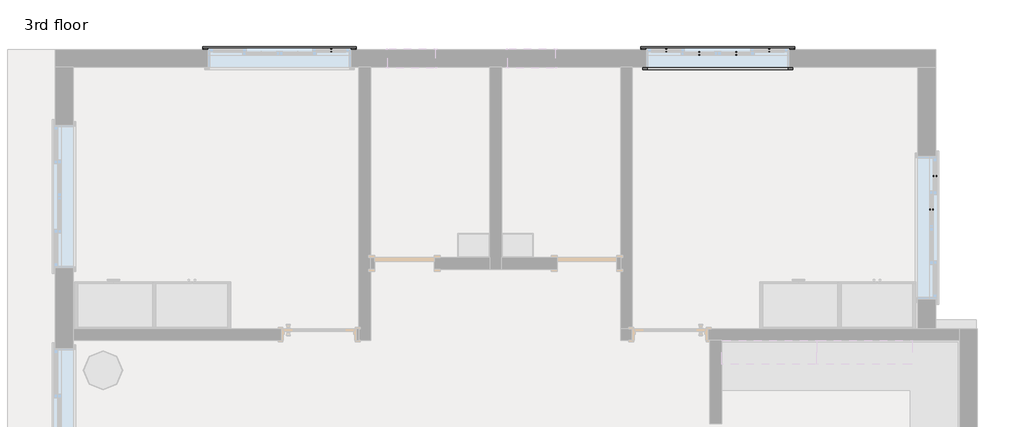
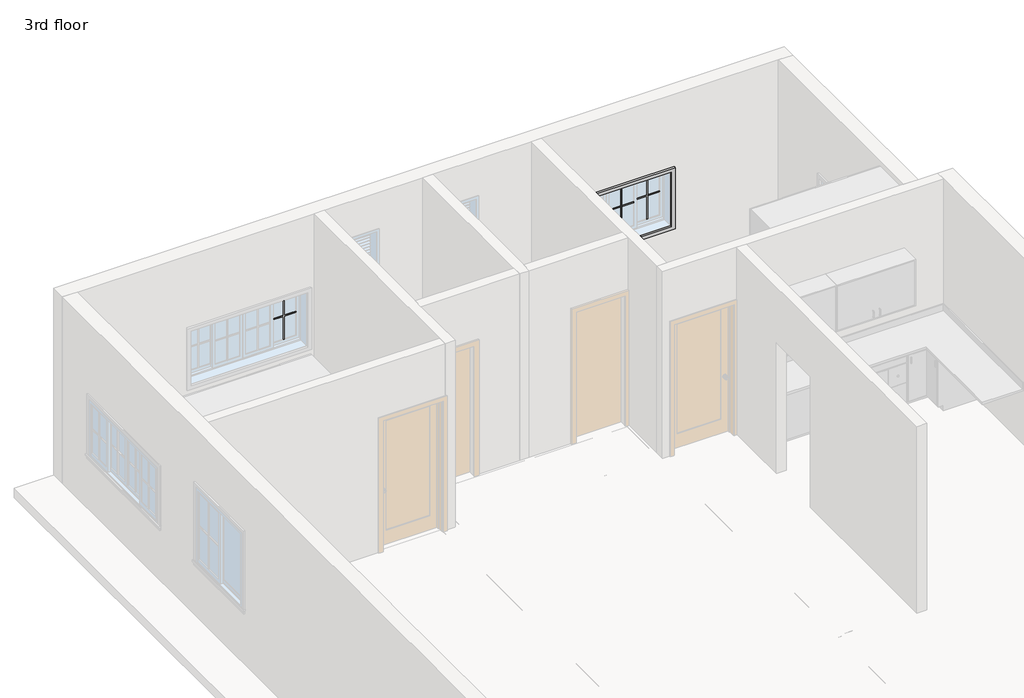
# One storey, part 4 of 4: 10 proxies.
"""IFC4 building model written with IfcOpenShell, lengths in millimetres."""

from ifc_helpers import new_model, si_unit, origin, place, context, project, spatial, transform, mapped, element, save
from components import muntin_pattern_2x2_muntin_pattern_2x2_31a16349, trim_window_exterior_flat_with_sill_3c945769, trim_window_interior_flat_picture_frame_0edfbaa2

model = new_model("IFC4")

# Units and contexts
model_context = context("Model", 3, world=origin())
ifc_project = project(units=[si_unit("LENGTHUNIT", "METRE", prefix="MILLI")], contexts=[model_context])

# Site, building, storey
site = spatial("IfcSite", under=ifc_project)
building = spatial("IfcBuilding", under=site)
storey = spatial("IfcBuildingStorey", under=building, Name="3rd floor", Elevation=10210.8)

# Proxies
placement = place(None, origin())
muntin_pattern_2x2_muntin_pattern_2x2_shape = muntin_pattern_2x2_muntin_pattern_2x2_31a16349(model_context)
element("IfcBuildingElementProxy", 1, Name="Muntin Pattern_2x2 : Muntin Pattern_2x2", ObjectType="Muntin Pattern_2x2 : Muntin Pattern_2x2", at=placement, inside=storey, context=model_context, shape_type="MappedRepresentation", body=[
    mapped(muntin_pattern_2x2_muntin_pattern_2x2_shape, transform((-9111.6124084, 10171.2711804, 11207.75), x_axis=(1.0, 0.0, 0.0), y_axis=(0.0, 1.0, 0.0), z_axis=(0.0, 0.0, 1.0))),
])
element("IfcBuildingElementProxy", 2, Name="Muntin Pattern_2x2 : Muntin Pattern_2x2", ObjectType="Muntin Pattern_2x2 : Muntin Pattern_2x2", at=placement, inside=storey, context=model_context, shape_type="MappedRepresentation", body=[
    mapped(muntin_pattern_2x2_muntin_pattern_2x2_shape, transform((-1374.1374084, 8555.1961804, 11207.75), x_axis=(0.0, -1.0, 0.0), y_axis=(1.0, 0.0, 0.0), z_axis=(0.0, 0.0, 1.0))),
])
element("IfcBuildingElementProxy", 3, Name="Muntin Pattern_2x2 : Muntin Pattern_2x2", ObjectType="Muntin Pattern_2x2 : Muntin Pattern_2x2", at=placement, inside=storey, context=model_context, shape_type="MappedRepresentation", body=[
    mapped(muntin_pattern_2x2_muntin_pattern_2x2_shape, transform((-1418.5874084, 8129.7461804, 11207.75), x_axis=(0.0, -1.0, 0.0), y_axis=(1.0, 0.0, 0.0), z_axis=(0.0, 0.0, 1.0))),
])
element("IfcBuildingElementProxy", 4, Name="Muntin Pattern_2x2 : Muntin Pattern_2x2", ObjectType="Muntin Pattern_2x2 : Muntin Pattern_2x2", at=placement, inside=storey, context=model_context, shape_type="MappedRepresentation", body=[
    mapped(muntin_pattern_2x2_muntin_pattern_2x2_shape, transform((-4819.0124084, 10171.2711804, 11207.75), x_axis=(1.0, 0.0, 0.0), y_axis=(0.0, 1.0, 0.0), z_axis=(0.0, 0.0, 1.0))),
])
element("IfcBuildingElementProxy", 5, Name="Muntin Pattern_2x2 : Muntin Pattern_2x2", ObjectType="Muntin Pattern_2x2 : Muntin Pattern_2x2", at=placement, inside=storey, context=model_context, shape_type="MappedRepresentation", body=[
    mapped(muntin_pattern_2x2_muntin_pattern_2x2_shape, transform((-4393.5624084, 10126.8211804, 11207.75), x_axis=(1.0, 0.0, 0.0), y_axis=(0.0, 1.0, 0.0), z_axis=(0.0, 0.0, 1.0))),
])
element("IfcBuildingElementProxy", 6, Name="Muntin Pattern_2x2 : Muntin Pattern_2x2", ObjectType="Muntin Pattern_2x2 : Muntin Pattern_2x2", at=placement, inside=storey, context=model_context, shape_type="MappedRepresentation", body=[
    mapped(muntin_pattern_2x2_muntin_pattern_2x2_shape, transform((-3923.6624084, 10126.8211804, 11207.75), x_axis=(1.0, 0.0, 0.0), y_axis=(0.0, 1.0, 0.0), z_axis=(0.0, 0.0, 1.0))),
])
element("IfcBuildingElementProxy", 7, Name="Muntin Pattern_2x2 : Muntin Pattern_2x2", ObjectType="Muntin Pattern_2x2 : Muntin Pattern_2x2", at=placement, inside=storey, context=model_context, shape_type="MappedRepresentation", body=[
    mapped(muntin_pattern_2x2_muntin_pattern_2x2_shape, transform((-3498.2124084, 10171.2711804, 11207.75), x_axis=(1.0, 0.0, 0.0), y_axis=(0.0, 1.0, 0.0), z_axis=(0.0, 0.0, 1.0))),
])
trim_window_exterior_flat_with_sill_shape = trim_window_exterior_flat_with_sill_3c945769(model_context)
element("IfcBuildingElementProxy", 8, Name="Trim-Window-Exterior-Flat : with Sill", ObjectType="Trim-Window-Exterior-Flat : with Sill", at=placement, inside=storey, context=model_context, shape_type="MappedRepresentation", body=[
    mapped(trim_window_exterior_flat_with_sill_shape, transform((-9772.0124084, 10180.7961804, 12039.6), x_axis=(-1.0, 0.0, 0.0), y_axis=(0.0, 0.0, 1.0), z_axis=(0.0, 1.0, 0.0))),
])
element("IfcBuildingElementProxy", 9, Name="Trim-Window-Exterior-Flat : with Sill", ObjectType="Trim-Window-Exterior-Flat : with Sill", at=placement, inside=storey, context=model_context, shape_type="MappedRepresentation", body=[
    mapped(trim_window_exterior_flat_with_sill_shape, transform((-4158.6124084, 10180.7961804, 12039.6), x_axis=(-1.0, 0.0, 0.0), y_axis=(0.0, 0.0, 1.0), z_axis=(0.0, 1.0, 0.0))),
])
trim_window_interior_flat_picture_frame_shape = trim_window_interior_flat_picture_frame_0edfbaa2(model_context)
element("IfcBuildingElementProxy", 10, Name="Trim-Window-Interior-Flat : Picture Frame", ObjectType="Trim-Window-Interior-Flat : Picture Frame", at=placement, inside=storey, context=model_context, shape_type="MappedRepresentation", body=[
    mapped(trim_window_interior_flat_picture_frame_shape, transform((-4158.6124084, 9952.1961804, 12039.6), x_axis=(1.0, 0.0, 0.0), y_axis=(0.0, 0.0, 1.0), z_axis=(0.0, -1.0, 0.0))),
])

save(model, "model.ifc")

# Revit data of these elements
# Type "Muntin Pattern_2x2 : Muntin Pattern_2x2"
#   Width [instance default] = 4' - 0"
#   Thickness = 0' - 0 1/2"
#   Height [instance default] = 4' - 0"
#   Distance = 0' - 0 3/4"
#   Interior Material [instance default] = none
#   Exterior Material [instance default] = none
#   Default Elevation = 0
# Type "Trim-Window-Exterior-Flat : with Sill"
#   Trim Width = 0' - 2 1/4"
#   Trim Thickness_Picture Frame = 0' - 1 1/4"
#   Trim Thickness_with Sill = 0' - 0 3/4"
#   Sill Thickness = 0' - 1 1/4"
#   Opening Width [instance default] = 2' - 0"
#   Opening Height [instance default] = 3' - 0"
#   Default Elevation = 4' - 0"
#   Sill = yes
#   Picture Frame = no
#   Trim Material [instance default] = none
# Type "Trim-Window-Interior-Flat : Picture Frame"
#   Trim Thickness_Picture Frame = 0' - 1 1/4"
#   Trim Width = 0' - 2 1/4"
#   Trim Thickness_with Sill = 0' - 0 3/4"
#   Sill Thickness = 0' - 1 1/4"
#   Opening Width [instance default] = 2' - 0"
#   Opening Height [instance default] = 3' - 0"
#   Default Elevation = 4' - 0"
#   Sill = no
#   Picture Frame = yes
#   Trim Material [instance default] = none
# Elements 1, 2, 3, 4, 5, 6, 7 (IfcBuildingElementProxy, "Muntin Pattern_2x2 : Muntin Pattern_2x2")
#   Width = 1' - 3"
#   Height = 2' - 6 1/4"
#   Interior Material = Wood - Stained
#   Exterior Material = Clad - White
#   Phase Created = New Construction
#   Materials on its faces: "Clad - White", "Wood - Stained"
# Elements 8, 9 (IfcBuildingElementProxy, "Trim-Window-Exterior-Flat : with Sill")
#   Opening Width = 6' - 0"
#   Opening Height = 3' - 0"
#   Trim Material = Clad - White
#   Phase Created = New Construction
#   Materials on its faces: "Clad - White"
# Element 10 (IfcBuildingElementProxy, "Trim-Window-Interior-Flat : Picture Frame")
#   Opening Width = 6' - 0"
#   Opening Height = 3' - 0"
#   Trim Material = Wood - Stained
#   Phase Created = New Construction
#   Materials on its faces: "Wood - Stained"
# Materials
#   "Clad - White": class "Wood", colour RGB 242 242 238, transparency 0, Cost = 0
#   "Wood - Stained": class "Wood", colour RGB 224 178 126, transparency 0, Cost = 0
